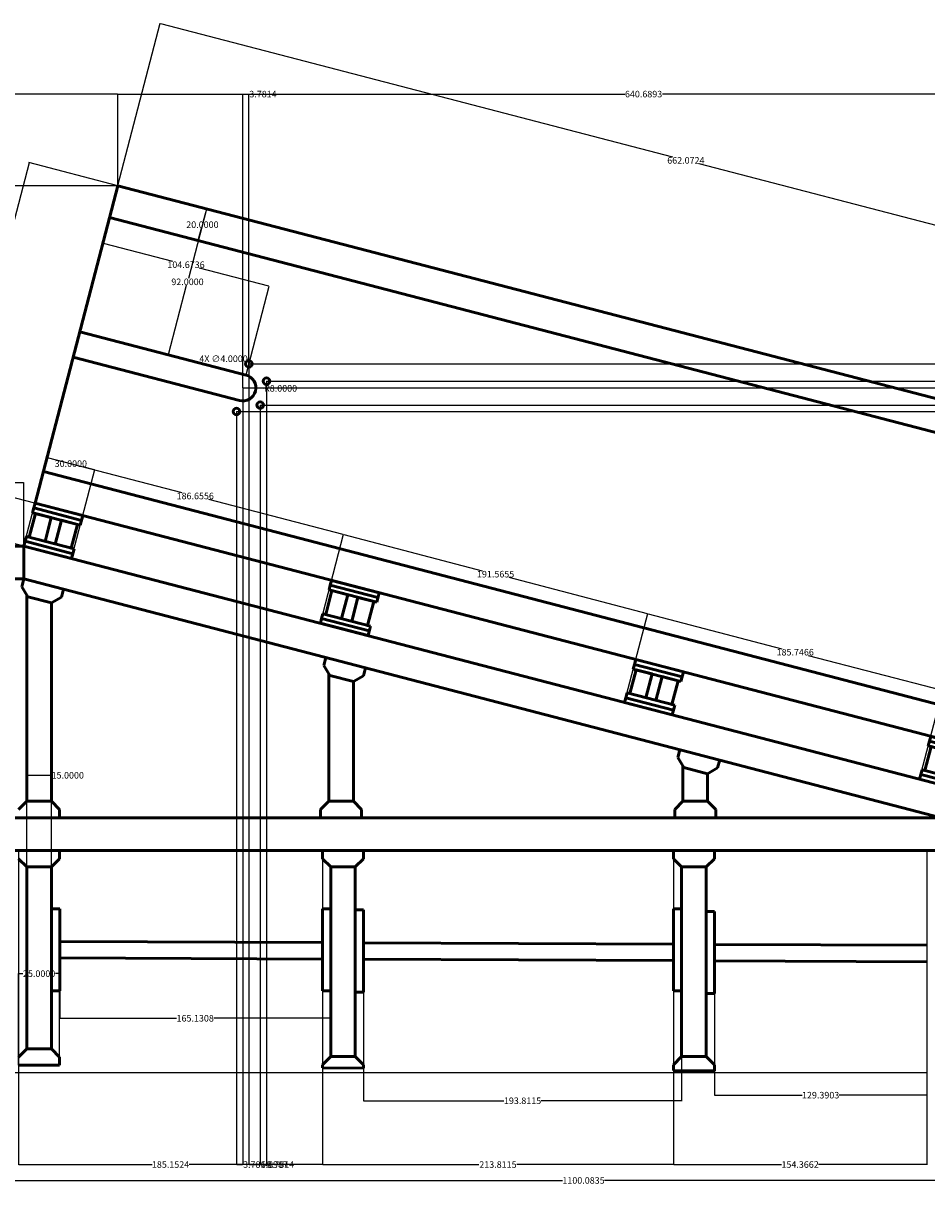
# Model space of a CAD drawing. Units: millimetres. Extents: x -54 to 1187, y -193 to 515.
# Tile 2 of 3: x 222 to 773, y -193 to 515. Entities that reach past the tile are written whole.
import ezdxf

# ---------------------------------------------------------------- set-up
doc = ezdxf.new("R2010")
doc.units = ezdxf.units.MM
doc.header["$MEASUREMENT"] = 0
doc.layers.add('M-DIMS', color=2, linetype='Continuous', lineweight=25)
doc.layers.add('M-OUTL', color=7, linetype='Continuous', lineweight=50)
doc.styles.get("Standard").update_dxf_attribs({"font": 'arial.ttf'})
doc.dimstyles.get("Standard").update_dxf_attribs({"dimtxt": 4, "dimasz": 0.18, "dimexe": 0.18, "dimexo": 0.0625, "dimgap": 0.09, "dimtad": 0, "dimtih": 1, "dimtoh": 1, "dimdec": 4, "dimzin": 0, "dimdsep": 46, "dimtxsty": 'Standard', "dimcen": 0.09, "dimclrd": 3, "dimclre": 3, "dimclrt": 1, "dimadec": 0, "dimazin": 0, "dimtfac": 1, "dimtdec": 4, "dimtofl": 0, "dimtmove": 0, "dimatfit": 3, "dimfxl": 1, "dimtolj": 1, "dimtzin": 0, "dimarcsym": 0})

# ---------------------------------------------------------------- blocks, each defined once
blk = doc.blocks.new('*D1')
at = {"layer": 'Defpoints', "color": 0, "transparency": 16777216}
for p in [(13.68, 20.33), (1113.76, 20.33), (1113.76, -190.81)]:
    blk.add_point(p, dxfattribs=at)
at = {"layer": 'M-DIMS', "color": 0, "lineweight": -2, "transparency": 16777216}
for p, q in [((13.68, 20.27), (13.68, -190.99)), ((1113.76, 20.27), (1113.76, -190.99)), ((13.86, -190.81), (550.84, -190.81)), ((1113.58, -190.81), (576.6, -190.81))]:
    blk.add_line(p, q, dxfattribs=at)
at = {"layer": 'M-DIMS', "color": 0, "transparency": 16777216}
for points in [[(13.86, -190.78), (13.86, -190.84), (13.68, -190.81)], [(1113.58, -190.78), (1113.58, -190.84), (1113.76, -190.81)]]:
    blk.add_solid(points, dxfattribs=at)
at = {"layer": 'M-DIMS', "color": 0, "transparency": 16777216, "insert": (563.72, -190.81), "char_height": 4, "attachment_point": 5}
blk.add_mtext('\\A1;1100.0835', dxfattribs=at)
blk = doc.blocks.new('*D2')
at = {"layer": 'Defpoints', "color": 0, "transparency": 16777216}
for p in [(244.55, -55.15), (409.68, -57.46), (409.68, -91.94)]:
    blk.add_point(p, dxfattribs=at)
at = {"layer": 'M-DIMS', "color": 0, "lineweight": -2, "transparency": 16777216}
for p, q in [((244.55, -55.22), (244.55, -92.12)), ((409.68, -57.52), (409.68, -92.12)), ((244.73, -91.94), (315.8, -91.94)), ((409.5, -91.94), (338.43, -91.94))]:
    blk.add_line(p, q, dxfattribs=at)
at = {"layer": 'M-DIMS', "color": 0, "transparency": 16777216}
for points in [[(244.73, -91.91), (244.73, -91.97), (244.55, -91.94)], [(409.5, -91.91), (409.5, -91.97), (409.68, -91.94)]]:
    blk.add_solid(points, dxfattribs=at)
at = {"layer": 'M-DIMS', "color": 0, "transparency": 16777216, "insert": (327.11, -91.94), "char_height": 4, "attachment_point": 5}
blk.add_mtext('\\A1;165.1308', dxfattribs=at)
blk = doc.blocks.new('*D3')
at = {"layer": 'Defpoints', "color": 0, "transparency": 16777216}
for p in [(429.68, -55.95), (623.49, -55.95), (623.49, -142.23)]:
    blk.add_point(p, dxfattribs=at)
at = {"layer": 'M-DIMS', "color": 0, "lineweight": -2, "transparency": 16777216}
for p, q in [((429.68, -56.02), (429.68, -142.41)), ((623.49, -56.02), (623.49, -142.41)), ((429.86, -142.23), (515.26, -142.23)), ((623.31, -142.23), (537.91, -142.23))]:
    blk.add_line(p, q, dxfattribs=at)
at = {"layer": 'M-DIMS', "color": 0, "transparency": 16777216}
for points in [[(429.86, -142.2), (429.86, -142.26), (429.68, -142.23)], [(623.31, -142.2), (623.31, -142.26), (623.49, -142.23)]]:
    blk.add_solid(points, dxfattribs=at)
at = {"layer": 'M-DIMS', "color": 0, "transparency": 16777216, "insert": (526.58, -142.23), "char_height": 4, "attachment_point": 5}
blk.add_mtext('\\A1;193.8115', dxfattribs=at)
blk = doc.blocks.new('*D4')
at = {"layer": 'Defpoints', "color": 0, "transparency": 16777216}
for p in [(643.49, -51.86), (772.88, -51.86), (772.88, -138.82)]:
    blk.add_point(p, dxfattribs=at)
at = {"layer": 'M-DIMS', "color": 0, "lineweight": -2, "transparency": 16777216}
for p, q in [((643.49, -51.92), (643.49, -139)), ((772.88, -51.92), (772.88, -139)), ((643.67, -138.82), (696.87, -138.82)), ((772.7, -138.82), (719.5, -138.82))]:
    blk.add_line(p, q, dxfattribs=at)
at = {"layer": 'M-DIMS', "color": 0, "transparency": 16777216}
for points in [[(643.67, -138.79), (643.67, -138.85), (643.49, -138.82)], [(772.7, -138.79), (772.7, -138.85), (772.88, -138.82)]]:
    blk.add_solid(points, dxfattribs=at)
at = {"layer": 'M-DIMS', "color": 0, "transparency": 16777216, "insert": (708.19, -138.82), "char_height": 4, "attachment_point": 5}
blk.add_mtext('\\A1;129.3903', dxfattribs=at)
blk = doc.blocks.new('*D5')
at = {"layer": 'Defpoints', "color": 0, "transparency": 16777216}
for p in [(222.75, 234.49), (22.75, 195.91), (222.75, 195.91)]:
    blk.add_point(p, dxfattribs=at)
at = {"layer": 'M-DIMS', "color": 0, "lineweight": -2, "transparency": 16777216}
for p, q in [((22.75, 195.98), (22.75, 234.67)), ((22.93, 234.49), (111.22, 234.49)), ((222.57, 234.49), (134.28, 234.49)), ((222.75, 195.98), (222.75, 234.67))]:
    blk.add_line(p, q, dxfattribs=at)
at = {"layer": 'M-DIMS', "color": 0, "transparency": 16777216}
for points in [[(22.93, 234.52), (22.93, 234.46), (22.75, 234.49)], [(222.57, 234.52), (222.57, 234.46), (222.75, 234.49)]]:
    blk.add_solid(points, dxfattribs=at)
at = {"layer": 'M-DIMS', "color": 0, "transparency": 16777216, "insert": (122.75, 234.49), "char_height": 4, "attachment_point": 5}
blk.add_mtext('\\A1;200.0000', dxfattribs=at)
blk = doc.blocks.new('*D6')
at = {"layer": 'Defpoints', "color": 0, "transparency": 16777216}
for p in [(279.97, 415.58), (946.42, 347.55), (920.66, 248.68)]:
    blk.add_point(p, dxfattribs=at)
at = {"layer": 'M-DIMS', "color": 0, "lineweight": -2, "transparency": 16777216}
for p, q in [((279.99, 415.64), (305.78, 514.63)), ((305.91, 514.41), (617.89, 433.14)), ((946.25, 347.6), (634.26, 428.87)), ((920.68, 248.74), (946.47, 347.73))]:
    blk.add_line(p, q, dxfattribs=at)
at = {"layer": 'M-DIMS', "color": 0, "transparency": 16777216}
for points in [[(305.91, 514.44), (305.9, 514.38), (305.73, 514.46)], [(946.26, 347.63), (946.24, 347.57), (946.42, 347.55)]]:
    blk.add_solid(points, dxfattribs=at)
at = {"layer": 'M-DIMS', "color": 0, "transparency": 16777216, "insert": (626.08, 431.01), "char_height": 4, "attachment_point": 5}
blk.add_mtext('\\A1;662.0724', dxfattribs=at)
blk = doc.blocks.new('ROLLER-BEARING-UNIT')
for p, q in [((5.29, 27.88), (6.05, 30.79)), ((6.81, 33.69), (6.05, 30.79)), ((6.05, 30.79), (35.08, 23.23)), ((35.84, 26.13), (6.81, 33.69)), ((3.24, 12.92), (7.02, 27.44)), ((5.29, 27.88), (34.33, 20.32)), ((7.02, 27.44), (16.7, 24.91)), ((16.7, 24.91), (12.91, 10.4)), ((22.91, 23.3), (19.12, 8.78)), ((32.58, 20.78), (22.91, 23.3)), ((34.33, 20.32), (35.84, 26.13)), ((28.8, 6.26), (32.58, 20.78)), ((0, 7.56), (0.76, 10.47)), ((0, 7.56), (29.03, 0)), ((1.51, 13.37), (0.76, 10.47)), ((0.76, 10.47), (29.79, 2.9)), ((30.54, 5.81), (1.51, 13.37)), ((30.54, 5.81), (28.8, 6.26)), ((29.03, 0), (30.54, 5.81)), ((29.79, 2.9), (29.03, 0))]:
    blk.add_line(p, q)
blk = doc.blocks.new('FLANGE-PLATE')
for p, q in [((0, 50), (0, 0)), ((5, 50), (0, 50)), ((5, 0), (5, 50)), ((0, 0), (5, 0))]:
    blk.add_line(p, q)
blk = doc.blocks.new('*D13')
at = {"layer": 'Defpoints', "color": 0, "transparency": 16777216}
for p in [(-42.17, 415.58), (279.97, 415.58), (772.86, -125.25)]:
    blk.add_point(p, dxfattribs=at)
at = {"layer": 'M-DIMS', "color": 3, "lineweight": -2, "transparency": 16777216}
for p, q in [((279.91, 415.58), (-42.35, 415.58)), ((-42.17, 415.4), (-42.17, 147.3)), ((-42.17, -125.07), (-42.17, 143.03)), ((772.79, -125.25), (-42.35, -125.25))]:
    blk.add_line(p, q, dxfattribs=at)
at = {"layer": 'M-DIMS', "color": 3, "transparency": 16777216}
for points in [[(-42.2, 415.4), (-42.14, 415.4), (-42.17, 415.58)], [(-42.2, -125.07), (-42.14, -125.07), (-42.17, -125.25)]]:
    blk.add_solid(points, dxfattribs=at)
at = {"layer": 'M-DIMS', "color": 1, "transparency": 16777216, "insert": (-42.17, 145.16), "char_height": 4, "attachment_point": 5}
blk.add_mtext('\\A1;540.8329', dxfattribs=at)
blk = doc.blocks.new('*D16')
at = {"layer": 'Defpoints', "color": 0, "transparency": 16777216}
for p in [(219.53, 10.33), (404.68, 10.33), (404.68, -181.1)]:
    blk.add_point(p, dxfattribs=at)
at = {"layer": 'M-DIMS', "color": 3, "lineweight": -2, "transparency": 16777216}
for p, q in [((219.53, 10.27), (219.53, -181.28)), ((404.68, 10.27), (404.68, -181.28)), ((219.71, -181.1), (300.8, -181.1)), ((404.5, -181.1), (323.41, -181.1))]:
    blk.add_line(p, q, dxfattribs=at)
at = {"layer": 'M-DIMS', "color": 3, "transparency": 16777216}
for points in [[(219.71, -181.07), (219.71, -181.13), (219.53, -181.1)], [(404.5, -181.07), (404.5, -181.13), (404.68, -181.1)]]:
    blk.add_solid(points, dxfattribs=at)
at = {"layer": 'M-DIMS', "color": 1, "transparency": 16777216, "insert": (312.1, -181.1), "char_height": 4, "attachment_point": 5}
blk.add_mtext('\\A1;185.1524', dxfattribs=at)
blk = doc.blocks.new('*D17')
at = {"layer": 'Defpoints', "color": 0, "transparency": 16777216}
for p in [(404.68, 10.33), (618.49, 10.33), (618.49, -181.1)]:
    blk.add_point(p, dxfattribs=at)
at = {"layer": 'M-DIMS', "color": 3, "lineweight": -2, "transparency": 16777216}
for p, q in [((404.68, 10.27), (404.68, -181.28)), ((618.49, 10.27), (618.49, -181.28)), ((404.86, -181.1), (500.03, -181.1)), ((618.31, -181.1), (523.13, -181.1))]:
    blk.add_line(p, q, dxfattribs=at)
at = {"layer": 'M-DIMS', "color": 3, "transparency": 16777216}
for points in [[(404.86, -181.07), (404.86, -181.13), (404.68, -181.1)], [(618.31, -181.07), (618.31, -181.13), (618.49, -181.1)]]:
    blk.add_solid(points, dxfattribs=at)
at = {"layer": 'M-DIMS', "color": 1, "transparency": 16777216, "insert": (511.58, -181.1), "char_height": 4, "attachment_point": 5}
blk.add_mtext('\\A1;213.8115', dxfattribs=at)
blk = doc.blocks.new('*D18')
at = {"layer": 'Defpoints', "color": 0, "transparency": 16777216}
for p in [(618.49, 10.33), (772.86, 10.33), (772.86, -181.1)]:
    blk.add_point(p, dxfattribs=at)
at = {"layer": 'M-DIMS', "color": 3, "lineweight": -2, "transparency": 16777216}
for p, q in [((618.49, 10.27), (618.49, -181.28)), ((772.86, 10.27), (772.86, -181.28)), ((618.67, -181.1), (684.38, -181.1)), ((772.68, -181.1), (706.97, -181.1))]:
    blk.add_line(p, q, dxfattribs=at)
at = {"layer": 'M-DIMS', "color": 3, "transparency": 16777216}
for points in [[(618.67, -181.07), (618.67, -181.13), (618.49, -181.1)], [(772.68, -181.07), (772.68, -181.13), (772.86, -181.1)]]:
    blk.add_solid(points, dxfattribs=at)
at = {"layer": 'M-DIMS', "color": 1, "transparency": 16777216, "insert": (695.67, -181.1), "char_height": 4, "attachment_point": 5}
blk.add_mtext('\\A1;154.3662', dxfattribs=at)
blk = doc.blocks.new('*D26')
at = {"layer": 'Defpoints', "color": 0, "transparency": 16777216}
for p in [(244.53, -64.74), (219.53, -120.59), (244.53, -120.59)]:
    blk.add_point(p, dxfattribs=at)
at = {"layer": 'M-DIMS', "color": 3, "lineweight": -2, "transparency": 16777216}
for p, q in [((219.53, -120.53), (219.53, -64.56)), ((219.71, -64.74), (222.05, -64.74)), ((244.35, -64.74), (242, -64.74)), ((244.53, -120.53), (244.53, -64.56))]:
    blk.add_line(p, q, dxfattribs=at)
at = {"layer": 'M-DIMS', "color": 3, "transparency": 16777216}
for points in [[(219.71, -64.71), (219.71, -64.77), (219.53, -64.74)], [(244.35, -64.71), (244.35, -64.77), (244.53, -64.74)]]:
    blk.add_solid(points, dxfattribs=at)
at = {"layer": 'M-DIMS', "color": 1, "transparency": 16777216, "insert": (232.03, -64.74), "char_height": 4, "attachment_point": 5}
blk.add_mtext('\\A1;25.0000', dxfattribs=at)
blk = doc.blocks.new('*D27')
at = {"layer": 'Defpoints', "color": 0, "transparency": 16777216}
for p in [(239.53, 56.18), (224.53, 0.33), (239.53, 0.33)]:
    blk.add_point(p, dxfattribs=at)
at = {"layer": 'M-DIMS', "color": 3, "lineweight": -2, "transparency": 16777216}
for p, q in [((224.53, 0.39), (224.53, 56.36)), ((224.71, 56.18), (239.35, 56.18)), ((239.53, 0.39), (239.53, 56.36)), ((239.53, 56.18), (239.71, 56.18))]:
    blk.add_line(p, q, dxfattribs=at)
at = {"layer": 'M-DIMS', "color": 3, "transparency": 16777216}
for points in [[(224.71, 56.21), (224.71, 56.15), (224.53, 56.18)], [(239.35, 56.21), (239.35, 56.15), (239.53, 56.18)]]:
    blk.add_solid(points, dxfattribs=at)
at = {"layer": 'M-DIMS', "color": 1, "transparency": 16777216, "insert": (249.46, 56.18), "char_height": 4, "attachment_point": 5}
blk.add_mtext('\\A1;15.0000', dxfattribs=at)
blk = doc.blocks.new('*D28')
at = {"layer": 'Defpoints', "color": 0, "transparency": 16777216}
for p in [(279.97, 471.43), (279.97, 415.58), (22.75, 195.91)]:
    blk.add_point(p, dxfattribs=at)
at = {"layer": 'M-DIMS', "color": 3, "lineweight": -2, "transparency": 16777216}
for p, q in [((22.75, 195.98), (22.75, 471.61)), ((22.93, 471.43), (139.83, 471.43)), ((279.79, 471.43), (162.9, 471.43)), ((279.97, 415.64), (279.97, 471.61))]:
    blk.add_line(p, q, dxfattribs=at)
at = {"layer": 'M-DIMS', "color": 3, "transparency": 16777216}
for points in [[(22.93, 471.46), (22.93, 471.4), (22.75, 471.43)], [(279.79, 471.46), (279.79, 471.4), (279.97, 471.43)]]:
    blk.add_solid(points, dxfattribs=at)
at = {"layer": 'M-DIMS', "color": 1, "transparency": 16777216, "insert": (151.36, 471.43), "char_height": 4, "attachment_point": 5}
blk.add_mtext('\\A1;257.2253', dxfattribs=at)
blk = doc.blocks.new('*D29')
at = {"layer": 'Defpoints', "color": 0, "transparency": 16777216}
for p in [(920.66, 471.43), (279.97, 415.58), (920.66, 248.68)]:
    blk.add_point(p, dxfattribs=at)
at = {"layer": 'M-DIMS', "color": 3, "lineweight": -2, "transparency": 16777216}
for p, q in [((279.97, 415.64), (279.97, 471.61)), ((280.15, 471.43), (588.81, 471.43)), ((920.48, 471.43), (611.83, 471.43)), ((920.66, 248.74), (920.66, 471.61))]:
    blk.add_line(p, q, dxfattribs=at)
at = {"layer": 'M-DIMS', "color": 3, "transparency": 16777216}
for points in [[(280.15, 471.46), (280.15, 471.4), (279.97, 471.43)], [(920.48, 471.46), (920.48, 471.4), (920.66, 471.43)]]:
    blk.add_solid(points, dxfattribs=at)
at = {"layer": 'M-DIMS', "color": 1, "transparency": 16777216, "insert": (600.32, 471.43), "char_height": 4, "attachment_point": 5}
blk.add_mtext('\\A1;640.6893', dxfattribs=at)
blk = doc.blocks.new('*D30')
at = {"layer": 'Defpoints', "color": 0, "transparency": 16777216}
for p in [(225.93, 429.66), (279.97, 415.58), (229.56, 222.04)]:
    blk.add_point(p, dxfattribs=at)
at = {"layer": 'M-DIMS', "color": 3, "lineweight": -2, "transparency": 16777216}
for p, q in [((225.88, 429.49), (201.27, 335.02)), ((279.91, 415.6), (225.75, 429.71)), ((175.56, 236.29), (200.16, 330.76)), ((229.5, 222.06), (175.34, 236.17))]:
    blk.add_line(p, q, dxfattribs=at)
at = {"layer": 'M-DIMS', "color": 3, "transparency": 16777216}
for points in [[(225.85, 429.49), (225.91, 429.48), (225.93, 429.66)], [(175.53, 236.3), (175.58, 236.29), (175.51, 236.12)]]:
    blk.add_solid(points, dxfattribs=at)
at = {"layer": 'M-DIMS', "color": 1, "transparency": 16777216, "insert": (200.72, 332.89), "char_height": 4, "attachment_point": 5}
blk.add_mtext('\\A1;200.0000', dxfattribs=at)
blk = doc.blocks.new('*D31')
at = {"layer": 'Defpoints', "color": 0, "transparency": 16777216}
for p in [(279.97, 415.58), (274.93, 396.23), (328.98, 382.15)]:
    blk.add_point(p, dxfattribs=at)
at = {"layer": 'M-DIMS', "color": 3, "lineweight": -2, "transparency": 16777216}
for p, q in [((280.04, 415.57), (334.2, 401.46)), ((333.98, 401.33), (332.06, 393.96)), ((274.99, 396.21), (329.15, 382.1)), ((329.02, 382.32), (330.94, 389.69))]:
    blk.add_line(p, q, dxfattribs=at)
at = {"layer": 'M-DIMS', "color": 3, "transparency": 16777216}
for points in [[(333.95, 401.34), (334, 401.32), (334.02, 401.5)], [(329, 382.33), (329.05, 382.31), (328.98, 382.15)]]:
    blk.add_solid(points, dxfattribs=at)
at = {"layer": 'M-DIMS', "color": 1, "transparency": 16777216, "insert": (331.5, 391.82), "char_height": 4, "attachment_point": 5}
blk.add_mtext('\\A1;20.0000', dxfattribs=at)
blk = doc.blocks.new('*D33')
at = {"layer": 'Defpoints', "color": 0, "transparency": 16777216}
for p in [(417.46, 202.93), (222.75, 195.91), (403.38, 148.88)]:
    blk.add_point(p, dxfattribs=at)
at = {"layer": 'M-DIMS', "color": 3, "lineweight": -2, "transparency": 16777216}
for p, q in [((222.77, 195.97), (236.87, 250.14)), ((237, 249.92), (318.95, 228.58)), ((417.28, 202.98), (335.33, 224.31)), ((403.4, 148.94), (417.5, 203.1))]:
    blk.add_line(p, q, dxfattribs=at)
at = {"layer": 'M-DIMS', "color": 3, "transparency": 16777216}
for points in [[(237, 249.94), (236.99, 249.89), (236.82, 249.96)], [(417.29, 203), (417.27, 202.95), (417.46, 202.93)]]:
    blk.add_solid(points, dxfattribs=at)
at = {"layer": 'M-DIMS', "color": 1, "transparency": 16777216, "insert": (327.14, 226.45), "char_height": 4, "attachment_point": 5}
blk.add_mtext('\\A1;186.6556', dxfattribs=at)
blk = doc.blocks.new('*D34')
at = {"layer": 'Defpoints', "color": 0, "transparency": 16777216}
for p in [(403.38, 148.88), (602.84, 154.64), (588.76, 100.59)]:
    blk.add_point(p, dxfattribs=at)
at = {"layer": 'M-DIMS', "color": 3, "lineweight": -2, "transparency": 16777216}
for p, q in [((403.4, 148.94), (417.51, 203.1)), ((417.64, 202.88), (501.97, 180.91)), ((602.67, 154.68), (518.34, 176.65)), ((588.78, 100.65), (602.89, 154.81))]:
    blk.add_line(p, q, dxfattribs=at)
at = {"layer": 'M-DIMS', "color": 3, "transparency": 16777216}
for points in [[(417.64, 202.91), (417.63, 202.85), (417.46, 202.93)], [(602.67, 154.71), (602.66, 154.65), (602.84, 154.64)]]:
    blk.add_solid(points, dxfattribs=at)
at = {"layer": 'M-DIMS', "color": 1, "transparency": 16777216, "insert": (510.15, 178.78), "char_height": 4, "attachment_point": 5}
blk.add_mtext('\\A1;191.5655', dxfattribs=at)
blk = doc.blocks.new('*D35')
at = {"layer": 'Defpoints', "color": 0, "transparency": 16777216}
for p in [(782.59, 107.81), (588.76, 100.59), (768.51, 53.76)]:
    blk.add_point(p, dxfattribs=at)
at = {"layer": 'M-DIMS', "color": 3, "lineweight": -2, "transparency": 16777216}
for p, q in [((588.78, 100.65), (602.89, 154.81)), ((603.02, 154.59), (684.53, 133.36)), ((782.41, 107.86), (700.9, 129.09)), ((768.52, 53.82), (782.63, 107.98))]:
    blk.add_line(p, q, dxfattribs=at)
at = {"layer": 'M-DIMS', "color": 3, "transparency": 16777216}
for points in [[(603.02, 154.62), (603.01, 154.56), (602.84, 154.64)], [(782.42, 107.88), (782.41, 107.83), (782.59, 107.81)]]:
    blk.add_solid(points, dxfattribs=at)
at = {"layer": 'M-DIMS', "color": 1, "transparency": 16777216, "insert": (692.71, 131.22), "char_height": 4, "attachment_point": 5}
blk.add_mtext('\\A1;185.7466', dxfattribs=at)
blk = doc.blocks.new('*D36')
at = {"layer": 'Defpoints', "color": 0, "transparency": 16777216}
for p in [(265.86, 242.4), (222.75, 195.91), (251.78, 188.35)]:
    blk.add_point(p, dxfattribs=at)
at = {"layer": 'M-DIMS', "color": 3, "lineweight": -2, "transparency": 16777216}
for p, q in [((222.77, 195.97), (236.87, 250.13)), ((237, 249.91), (243.15, 248.31)), ((251.8, 188.41), (265.91, 242.57)), ((265.69, 242.44), (259.53, 244.04))]:
    blk.add_line(p, q, dxfattribs=at)
at = {"layer": 'M-DIMS', "color": 3, "transparency": 16777216}
for points in [[(237.01, 249.94), (237, 249.88), (236.83, 249.96)], [(265.69, 242.47), (265.68, 242.41), (265.86, 242.4)]]:
    blk.add_solid(points, dxfattribs=at)
at = {"layer": 'M-DIMS', "color": 1, "transparency": 16777216, "insert": (251.34, 246.18), "char_height": 4, "attachment_point": 5}
blk.add_mtext('\\A1;30.0000', dxfattribs=at)
blk = doc.blocks.new('*D37')
at = {"layer": 'Defpoints', "color": 0, "transparency": 16777216}
for p in [(175.51, 236.12), (229.56, 222.04), (222.75, 195.91)]:
    blk.add_point(p, dxfattribs=at)
at = {"layer": 'M-DIMS', "color": 3, "lineweight": -2, "transparency": 16777216}
for p, q in [((175.46, 235.95), (172.66, 225.19)), ((229.5, 222.06), (175.34, 236.17)), ((168.75, 210.17), (171.55, 220.92)), ((222.69, 195.93), (168.53, 210.04))]:
    blk.add_line(p, q, dxfattribs=at)
at = {"layer": 'M-DIMS', "color": 3, "transparency": 16777216}
for points in [[(175.44, 235.95), (175.49, 235.94), (175.51, 236.12)], [(168.72, 210.17), (168.78, 210.16), (168.7, 209.99)]]:
    blk.add_solid(points, dxfattribs=at)
at = {"layer": 'M-DIMS', "color": 1, "transparency": 16777216, "insert": (172.11, 223.06), "char_height": 4, "attachment_point": 5}
blk.add_mtext('\\A1;27.0000', dxfattribs=at)
blk = doc.blocks.new('*D38')
at = {"layer": 'Defpoints', "color": 0, "transparency": 16777216}
for p in [(279.97, 415.58), (256.78, 326.55), (310.83, 312.47)]:
    blk.add_point(p, dxfattribs=at)
at = {"layer": 'M-DIMS', "color": 3, "lineweight": -2, "transparency": 16777216}
for p, q in [((280.04, 415.57), (334.2, 401.46)), ((333.98, 401.33), (322.98, 359.12)), ((310.87, 312.65), (321.87, 354.86)), ((256.84, 326.54), (311, 312.43))]:
    blk.add_line(p, q, dxfattribs=at)
at = {"layer": 'M-DIMS', "color": 3, "transparency": 16777216}
for points in [[(333.95, 401.34), (334, 401.32), (334.02, 401.5)], [(310.84, 312.65), (310.9, 312.64), (310.83, 312.47)]]:
    blk.add_solid(points, dxfattribs=at)
at = {"layer": 'M-DIMS', "color": 1, "transparency": 16777216, "insert": (322.42, 356.99), "char_height": 4, "attachment_point": 5}
blk.add_mtext('\\A1;92.0000', dxfattribs=at)
blk = doc.blocks.new('*D39')
at = {"layer": 'Defpoints', "color": 0, "transparency": 16777216}
for p in [(372.15, 354.21), (256.78, 326.55), (358.08, 300.17)]:
    blk.add_point(p, dxfattribs=at)
at = {"layer": 'M-DIMS', "color": 3, "lineweight": -2, "transparency": 16777216}
for p, q in [((256.8, 326.61), (270.91, 380.77)), ((271.04, 380.55), (313.32, 369.54)), ((371.98, 354.26), (329.7, 365.27)), ((358.09, 300.23), (372.2, 354.39))]:
    blk.add_line(p, q, dxfattribs=at)
at = {"layer": 'M-DIMS', "color": 3, "transparency": 16777216}
for points in [[(271.04, 380.58), (271.03, 380.52), (270.86, 380.6)], [(371.99, 354.29), (371.97, 354.23), (372.15, 354.21)]]:
    blk.add_solid(points, dxfattribs=at)
at = {"layer": 'M-DIMS', "color": 1, "transparency": 16777216, "insert": (321.51, 367.41), "char_height": 4, "attachment_point": 5}
blk.add_mtext('\\A1;104.6736', dxfattribs=at)
blk = doc.blocks.new('*D47')
at = {"layer": 'Defpoints', "color": 0, "transparency": 16777216}
for p in [(356.06, 292.42), (352.28, 277.91), (356.06, -181.1)]:
    blk.add_point(p, dxfattribs=at)
at = {"layer": 'M-DIMS', "color": 3, "lineweight": -2, "transparency": 16777216}
for p, q in [((356.06, 292.36), (356.06, -181.28)), ((352.28, 277.85), (352.28, -181.28)), ((352.46, -181.1), (355.88, -181.1)), ((356.06, -181.1), (356.24, -181.1))]:
    blk.add_line(p, q, dxfattribs=at)
at = {"layer": 'M-DIMS', "color": 3, "transparency": 16777216}
for points in [[(352.46, -181.07), (352.46, -181.13), (352.28, -181.1)], [(355.88, -181.07), (355.88, -181.13), (356.06, -181.1)]]:
    blk.add_solid(points, dxfattribs=at)
at = {"layer": 'M-DIMS', "color": 1, "transparency": 16777216, "insert": (364.62, -181.1), "char_height": 4, "attachment_point": 5}
blk.add_mtext('\\A1;3.7814', dxfattribs=at)
blk = doc.blocks.new('*D48')
at = {"layer": 'Defpoints', "color": 0, "transparency": 16777216}
for p in [(359.84, 471.43), (359.84, 306.94), (356.06, 292.42)]:
    blk.add_point(p, dxfattribs=at)
at = {"layer": 'M-DIMS', "color": 3, "lineweight": -2, "transparency": 16777216}
for p, q in [((356.06, 292.49), (356.06, 471.61)), ((356.24, 471.43), (359.66, 471.43)), ((359.84, 307), (359.84, 471.61)), ((359.84, 471.43), (360.02, 471.43))]:
    blk.add_line(p, q, dxfattribs=at)
at = {"layer": 'M-DIMS', "color": 3, "transparency": 16777216}
for points in [[(356.24, 471.46), (356.24, 471.4), (356.06, 471.43)], [(359.66, 471.46), (359.66, 471.4), (359.84, 471.43)]]:
    blk.add_solid(points, dxfattribs=at)
at = {"layer": 'M-DIMS', "color": 1, "transparency": 16777216, "insert": (368.4, 471.43), "char_height": 4, "attachment_point": 5}
blk.add_mtext('\\A1;3.7814', dxfattribs=at)
blk = doc.blocks.new('*D49')
at = {"layer": 'Defpoints', "color": 0, "transparency": 16777216}
for p in [(359.84, 306.94), (366.74, 281.89), (366.74, -181.1)]:
    blk.add_point(p, dxfattribs=at)
at = {"layer": 'M-DIMS', "color": 3, "lineweight": -2, "transparency": 16777216}
for p, q in [((359.84, 306.88), (359.84, -181.28)), ((366.74, 281.83), (366.74, -181.28)), ((360.02, -181.1), (366.56, -181.1)), ((366.74, -181.1), (366.92, -181.1))]:
    blk.add_line(p, q, dxfattribs=at)
at = {"layer": 'M-DIMS', "color": 3, "transparency": 16777216}
for points in [[(360.02, -181.07), (360.02, -181.13), (359.84, -181.1)], [(366.56, -181.07), (366.56, -181.13), (366.74, -181.1)]]:
    blk.add_solid(points, dxfattribs=at)
at = {"layer": 'M-DIMS', "color": 1, "transparency": 16777216, "insert": (375.32, -181.1), "char_height": 4, "attachment_point": 5}
blk.add_mtext('\\A1;6.8987', dxfattribs=at)
blk = doc.blocks.new('*D50')
at = {"layer": 'Defpoints', "color": 0, "transparency": 16777216}
for p in [(370.52, 296.41), (366.74, 281.89), (370.52, -181.1)]:
    blk.add_point(p, dxfattribs=at)
at = {"layer": 'M-DIMS', "color": 3, "lineweight": -2, "transparency": 16777216}
for p, q in [((370.52, 296.34), (370.52, -181.28)), ((366.74, 281.83), (366.74, -181.28)), ((366.92, -181.1), (370.34, -181.1)), ((370.52, -181.1), (370.7, -181.1))]:
    blk.add_line(p, q, dxfattribs=at)
at = {"layer": 'M-DIMS', "color": 3, "transparency": 16777216}
for points in [[(366.92, -181.07), (366.92, -181.13), (366.74, -181.1)], [(370.34, -181.07), (370.34, -181.13), (370.52, -181.1)]]:
    blk.add_solid(points, dxfattribs=at)
at = {"layer": 'M-DIMS', "color": 1, "transparency": 16777216, "insert": (379.08, -181.1), "char_height": 4, "attachment_point": 5}
blk.add_mtext('\\A1;3.7814', dxfattribs=at)
blk = doc.blocks.new('*D51')
at = {"layer": 'Defpoints', "color": 0, "transparency": 16777216}
for p in [(352.28, 277.91), (366.74, 281.89), (1169.7, 281.89)]:
    blk.add_point(p, dxfattribs=at)
at = {"layer": 'M-DIMS', "color": 3, "lineweight": -2, "transparency": 16777216}
for p, q in [((352.34, 277.91), (1169.88, 277.91)), ((366.8, 281.89), (1169.88, 281.89)), ((1169.7, 281.89), (1169.7, 282.07)), ((1169.7, 282.07), (1169.88, 282.07)), ((1169.7, 278.09), (1169.7, 281.71))]:
    blk.add_line(p, q, dxfattribs=at)
at = {"layer": 'M-DIMS', "color": 3, "transparency": 16777216}
for points in [[(1169.67, 281.71), (1169.73, 281.71), (1169.7, 281.89)], [(1169.67, 278.09), (1169.73, 278.09), (1169.7, 277.91)]]:
    blk.add_solid(points, dxfattribs=at)
at = {"layer": 'M-DIMS', "color": 1, "transparency": 16777216, "insert": (1178.26, 282.07), "char_height": 4, "attachment_point": 5}
blk.add_mtext('\\A1;3.9830', dxfattribs=at)
blk = doc.blocks.new('*D52')
at = {"layer": 'Defpoints', "color": 0, "transparency": 16777216}
for p in [(356.06, 292.42), (1169.7, 292.42), (366.74, 281.89)]:
    blk.add_point(p, dxfattribs=at)
at = {"layer": 'M-DIMS', "color": 3, "lineweight": -2, "transparency": 16777216}
for p, q in [((356.12, 292.42), (1169.88, 292.42)), ((1169.7, 292.24), (1169.7, 289.29)), ((1169.7, 282.07), (1169.7, 285.02)), ((366.8, 281.89), (1169.88, 281.89))]:
    blk.add_line(p, q, dxfattribs=at)
at = {"layer": 'M-DIMS', "color": 3, "transparency": 16777216}
for points in [[(1169.67, 292.24), (1169.73, 292.24), (1169.7, 292.42)], [(1169.67, 282.07), (1169.73, 282.07), (1169.7, 281.89)]]:
    blk.add_solid(points, dxfattribs=at)
at = {"layer": 'M-DIMS', "color": 1, "transparency": 16777216, "insert": (1169.7, 287.16), "char_height": 4, "attachment_point": 5}
blk.add_mtext('\\A1;10.5326', dxfattribs=at)
blk = doc.blocks.new('*D53')
at = {"layer": 'Defpoints', "color": 0, "transparency": 16777216}
for p in [(356.06, 292.42), (370.52, 296.41), (1169.7, 296.41)]:
    blk.add_point(p, dxfattribs=at)
at = {"layer": 'M-DIMS', "color": 3, "lineweight": -2, "transparency": 16777216}
for p, q in [((356.12, 292.42), (1169.88, 292.42)), ((370.58, 296.41), (1169.88, 296.41)), ((1169.7, 296.41), (1169.7, 296.59)), ((1169.7, 296.59), (1169.88, 296.59)), ((1169.7, 292.6), (1169.7, 296.23))]:
    blk.add_line(p, q, dxfattribs=at)
at = {"layer": 'M-DIMS', "color": 3, "transparency": 16777216}
for points in [[(1169.67, 296.23), (1169.73, 296.23), (1169.7, 296.41)], [(1169.67, 292.6), (1169.73, 292.6), (1169.7, 292.42)]]:
    blk.add_solid(points, dxfattribs=at)
at = {"layer": 'M-DIMS', "color": 1, "transparency": 16777216, "insert": (1178.26, 296.59), "char_height": 4, "attachment_point": 5}
blk.add_mtext('\\A1;3.9830', dxfattribs=at)
blk = doc.blocks.new('*D54')
at = {"layer": 'Defpoints', "color": 0, "transparency": 16777216}
for p in [(359.84, 306.94), (1169.7, 306.94), (370.52, 296.41)]:
    blk.add_point(p, dxfattribs=at)
at = {"layer": 'M-DIMS', "color": 3, "lineweight": -2, "transparency": 16777216}
for p, q in [((359.9, 306.94), (1169.88, 306.94)), ((1169.7, 306.76), (1169.7, 303.81)), ((1169.7, 296.59), (1169.7, 299.54)), ((370.58, 296.41), (1169.88, 296.41))]:
    blk.add_line(p, q, dxfattribs=at)
at = {"layer": 'M-DIMS', "color": 3, "transparency": 16777216}
for points in [[(1169.67, 306.76), (1169.73, 306.76), (1169.7, 306.94)], [(1169.67, 296.59), (1169.73, 296.59), (1169.7, 296.41)]]:
    blk.add_solid(points, dxfattribs=at)
at = {"layer": 'M-DIMS', "color": 1, "transparency": 16777216, "insert": (1169.7, 301.67), "char_height": 4, "attachment_point": 5}
blk.add_mtext('\\A1;10.5326', dxfattribs=at)
blk = doc.blocks.new('*D55')
at = {"layer": 'Defpoints', "color": 0, "transparency": 16777216}
for p in [(356.06, 292.42), (364.06, 292.2)]:
    blk.add_point(p, dxfattribs=at)
at = {"layer": 'M-DIMS', "color": 3, "lineweight": -2, "transparency": 16777216}
for p, q in [((355.97, 292.42), (356.15, 292.42)), ((356.06, 292.33), (356.06, 292.51)), ((368.85, 292.06), (364.24, 292.19))]:
    blk.add_line(p, q, dxfattribs=at)
at = {"layer": 'M-DIMS', "color": 3, "transparency": 16777216}
blk.add_solid([(364.24, 292.22), (364.23, 292.16), (364.06, 292.2)], dxfattribs=at)
at = {"layer": 'M-DIMS', "color": 1, "transparency": 16777216, "insert": (379.15, 292.06), "char_height": 4, "attachment_point": 5}
blk.add_mtext('\\A1;R8.0000', dxfattribs=at)
blk = doc.blocks.new('*D56')
at = {"layer": 'Defpoints', "color": 0, "transparency": 16777216}
for p in [(359.57, 308.92), (360.11, 304.96)]:
    blk.add_point(p, dxfattribs=at)
at = {"layer": 'M-DIMS', "color": 3, "lineweight": -2, "transparency": 16777216}
for p, q in [((359.23, 310.11), (359.41, 310.11)), ((359.41, 310.11), (359.55, 309.1)), ((359.75, 306.94), (359.93, 306.94)), ((359.84, 306.85), (359.84, 307.03))]:
    blk.add_line(p, q, dxfattribs=at)
at = {"layer": 'M-DIMS', "color": 3, "transparency": 16777216}
blk.add_solid([(359.58, 309.1), (359.52, 309.1), (359.57, 308.92)], dxfattribs=at)
at = {"layer": 'M-DIMS', "color": 1, "transparency": 16777216, "insert": (344.39, 310.11), "char_height": 4, "attachment_point": 5}
blk.add_mtext('\\A1;4X ∅4.0000', dxfattribs=at)

msp = doc.modelspace()

# ---------------------------------------------------------------- linework, layer by layer
at = {"layer": 'M-OUTL'}
for p, q in [((279.97484, 415.5813), (229.55607, 222.04074)), ((920.66417, 248.67693), (279.97484, 415.5813)), ((915.62229, 229.32287), (274.93296, 396.22724)), ((358.07512, 300.16508), (256.78221, 326.55264)), ((354.04162, 284.68183), (252.74871, 311.0694)), ((234.59795, 241.3948), (875.28728, 74.49042)), ((229.55607, 222.04074), (228.79979, 219.13763)), ((258.58716, 214.47792), (229.55607, 222.04074)), ((229.55607, 222.04074), (870.2454, 55.13637)), ((225.98662, 201.26973), (229.76803, 215.78527)), ((228.04351, 216.23452), (228.79979, 219.13763)), ((228.04351, 216.23452), (257.07459, 208.67171)), ((228.79979, 219.13763), (257.83088, 211.57482)), ((229.76803, 215.78527), (239.44505, 213.26433)), ((239.44505, 213.26433), (235.66365, 198.74879)), ((257.07459, 208.67171), (258.58716, 214.47792)), ((245.6557, 211.64641), (241.87429, 197.13087)), ((255.33273, 209.12548), (245.6557, 211.64641)), ((251.55132, 194.60993), (255.33273, 209.12548)), ((222.74954, 195.91276), (223.50582, 198.81587)), ((224.2621, 201.71898), (223.50582, 198.81587)), ((223.50582, 198.81587), (252.53691, 191.25306)), ((253.29319, 194.15617), (224.2621, 201.71898)), ((22.74954, 195.91276), (222.74954, 195.91276)), ((222.74954, 195.91276), (222.74954, 175.91276)), ((781.59027, 50.33057), (222.74954, 195.91276)), ((222.74954, 195.91276), (251.78062, 188.34995)), ((253.29319, 194.15617), (251.55132, 194.60993)), ((251.78062, 188.34995), (253.29319, 194.15617)), ((252.53691, 191.25306), (251.78062, 188.34995)), ((22.74954, 175.91276), (222.74954, 175.91276)), ((222.74954, 175.91276), (221.48907, 171.07425)), ((221.48907, 171.07425), (225.06992, 164.98609)), ((222.74954, 175.91276), (781.59027, 30.33057)), ((222.74954, 175.91276), (246.95604, 169.66414)), ((224.52653, 40.33057), (224.52653, 165.91276)), ((239.52653, 161.25453), (225.06992, 164.98609)), ((239.52653, 161.25453), (245.66195, 164.83451)), ((246.95604, 169.66414), (245.66195, 164.83451)), ((239.52653, 40.33057), (239.52653, 161.25453)), ((406.72839, 127.9849), (405.46792, 123.14638)), ((405.46792, 123.14638), (409.04877, 117.05822)), ((430.93489, 121.73627), (429.64079, 116.90664)), ((408.50538, 40.33057), (408.50538, 117.98209)), ((423.50538, 113.32666), (409.04877, 117.05822)), ((423.50538, 113.32666), (429.64079, 116.90664)), ((423.50538, 40.33057), (423.50538, 113.32666)), ((622.50168, 71.77433), (621.24122, 66.93582)), ((621.24122, 66.93582), (624.82207, 60.84766)), ((646.70819, 65.52571), (645.41409, 60.69608)), ((624.27868, 40.33057), (624.27868, 61.77153)), ((639.27868, 57.1161), (624.82207, 60.84766)), ((639.27868, 57.1161), (645.41409, 60.69608)), ((639.27868, 40.33057), (639.27868, 57.1161)), ((219.52653, 35.33057), (224.52653, 40.33057)), ((224.52653, 40.33057), (239.52653, 40.33057)), ((244.52653, 35.33057), (239.52653, 40.33057)), ((403.50538, 35.33057), (408.50538, 40.33057)), ((408.50538, 40.33057), (423.50538, 40.33057)), ((428.50538, 35.33057), (423.50538, 40.33057)), ((619.27868, 35.33057), (624.27868, 40.33057)), ((624.27868, 40.33057), (639.27868, 40.33057)), ((644.27868, 35.33057), (639.27868, 40.33057)), ((13.67803, 30.33057), (1013.67803, 30.33057)), ((244.52653, 35.33057), (244.52653, 30.33057)), ((403.50538, 30.33057), (403.50538, 35.33057)), ((428.50538, 35.33057), (428.50538, 30.33057)), ((619.27868, 30.33057), (619.27868, 35.33057)), ((644.27868, 35.33057), (644.27868, 30.33057)), ((1013.67803, 10.33057), (13.67803, 10.33057)), ((224.52653, 10.33057), (239.52653, 10.33057)), ((244.52653, 5.33057), (244.52653, 10.33057)), ((404.67896, 10.33057), (404.67896, 5.33057)), ((429.67896, 5.33057), (429.67896, 10.33057)), ((618.4905, 10.33057), (618.4905, 5.33057)), ((643.4905, 5.33057), (643.4905, 10.33057)), ((219.52653, 5.33057), (224.52653, 0.33057)), ((224.52653, -110.5934), (224.52653, 0.33057)), ((224.52653, 0.33057), (239.52653, 0.33057)), ((244.52653, 5.33057), (239.52653, 0.33057)), ((239.52653, -110.5934), (239.52653, 0.33057)), ((404.67896, 5.33057), (409.67896, 0.33057)), ((409.67896, -115.25163), (409.67896, 0.33057)), ((409.67896, 0.33057), (424.67896, 0.33057)), ((429.67896, 5.33057), (424.67896, 0.33057)), ((424.67896, -115.25163), (424.67896, 0.33057)), ((618.4905, 5.33057), (623.4905, 0.33057)), ((623.4905, -115.25163), (623.4905, 0.33057)), ((623.4905, 0.33057), (638.4905, 0.33057)), ((643.4905, 5.33057), (638.4905, 0.33057)), ((638.4905, -115.25163), (638.4905, 0.33057)), ((239.54816, -45.13146), (239.54816, -55.13142)), ((244.54816, -45.15309), (404.67896, -45.84591)), ((424.67896, -45.93244), (424.67896, -55.93253)), ((429.67896, -45.95407), (618.4905, -46.77098)), ((638.4905, -46.85751), (638.4905, -56.8576)), ((643.4905, -46.87914), (772.85666, -47.43885)), ((239.5049, -55.13137), (239.54816, -55.13156)), ((244.54816, -55.15319), (404.67896, -55.846)), ((429.67896, -55.95417), (618.4905, -56.77107)), ((643.4905, -56.87924), (772.85666, -57.43895)), ((219.52653, -115.5934), (224.52653, -110.5934)), ((224.52653, -110.5934), (239.52653, -110.5934)), ((244.52653, -115.5934), (239.52653, -110.5934)), ((244.52653, -115.5934), (244.52653, -120.5934)), ((404.67896, -120.25163), (409.67896, -115.25163)), ((404.67896, -122.08473), (404.67896, -120.25163)), ((409.67896, -115.25163), (424.67896, -115.25163)), ((429.67896, -120.25163), (424.67896, -115.25163)), ((429.67896, -120.25163), (429.67896, -122.2861)), ((618.4905, -120.25163), (623.4905, -115.25163)), ((618.4905, -123.8069), (618.4905, -120.25163)), ((623.4905, -115.25163), (638.4905, -115.25163)), ((643.4905, -120.25163), (638.4905, -115.25163)), ((643.4905, -120.25163), (643.4905, -124.00827)), ((219.52653, -120.5934), (244.52653, -120.5934)), ((404.67896, -122.08473), (429.67896, -122.2861)), ((618.4905, -123.8069), (643.4905, -124.00827))]:
    msp.add_line(p, q, dxfattribs=at)
for centre in [(359.83977, 306.939), (370.5199, 296.40643), (366.73849, 281.89089), (352.27696, 277.90791)]:
    msp.add_circle(centre, 2, dxfattribs=at)
msp.add_arc((356.05837, 292.42346), 8, 255.39855107, 75.39855107, dxfattribs=at)

# ---------------------------------------------------------------- block references
for name, p in [('ROLLER-BEARING-UNIT', (403.383, 141.319)), ('ROLLER-BEARING-UNIT', (588.76146, 93.02652)), ('ROLLER-BEARING-UNIT', (768.50893, 46.20096)), ('FLANGE-PLATE', (239.548, -75.131))]:
    msp.add_blockref(name, p, dxfattribs=at)
at = {"layer": 'M-OUTL', "rotation": 180}
for p in [(409.67912, -25.13188), (429.67912, -25.93293), (623.49066, -25.13188), (643.49066, -26.85799)]:
    msp.add_blockref('FLANGE-PLATE', p, dxfattribs=at)

# ---------------------------------------------------------------- dimensions: what is measured, and where the dimension line sits
at = {"layer": 'M-DIMS'}
dim = msp.add_aligned_dim(p1=(279.97484, 415.5813), p2=(920.66417, 248.67693), distance=102.17685, dimstyle='Standard', override={"dimclrd": 0, "dimclre": 0, "dimclrt": 0}, dxfattribs=at)
dim.commit()
dim.dimension.update_dxf_attribs({"geometry": '*D6', "text_midpoint": (626.07766, 431.00594)})
for base, p1, p2, override, picture, middle in [((279.97484, 471.4313), (22.74954, 195.91276), (279.97484, 415.5813), {"dimdec": 4, "dimlfac": 1, "dimrnd": 0, "dimzin": 0, "dimdsep": 46, "dimlunit": 2}, '*D28', (151.36219, 471.4313)), ((920.66417, 471.4313), (279.97484, 415.5813), (920.66417, 248.67693), {"dimdec": 4, "dimlfac": 1, "dimrnd": 0, "dimzin": 0, "dimdsep": 46, "dimlunit": 2}, '*D29', (600.3195, 471.4313)), ((359.83977, 471.4313), (356.05837, 292.42346), (359.83977, 306.939), {"dimdec": 4, "dimlfac": 1, "dimrnd": 0, "dimzin": 0, "dimdsep": 46, "dimlunit": 2}, '*D48', (368.40309, 471.4313)), ((366.73849, -181.10163), (359.83977, 306.939), (366.73849, 281.89089), {"dimdec": 4, "dimlfac": 1, "dimrnd": 0, "dimzin": 0, "dimdsep": 46, "dimlunit": 2}, '*D49', (375.32227, -181.10163)), ((356.05837, -181.10163), (352.27696, 277.90792), (356.05837, 292.42346), {"dimdec": 4, "dimlfac": 1, "dimrnd": 0, "dimzin": 0, "dimdsep": 46, "dimlunit": 2}, '*D47', (364.62168, -181.10163)), ((370.5199, -181.10163), (366.73849, 281.89089), (370.5199, 296.40643), {"dimdec": 4, "dimlfac": 1, "dimrnd": 0, "dimzin": 0, "dimdsep": 46, "dimlunit": 2}, '*D50', (379.08321, -181.10163)), ((222.74954, 234.49469), (22.74954, 195.91276), (222.74954, 195.91276), {"dimclrd": 0, "dimclre": 0, "dimclrt": 0}, '*D5', (122.74954, 234.49469)), ((239.52653, 56.18057), (224.52653, 0.33057), (239.52653, 0.33057), {"dimdec": 4, "dimlfac": 1, "dimrnd": 0, "dimzin": 0, "dimdsep": 46, "dimlunit": 2}, '*D27', (249.4582, 56.18057)), ((1113.76153, -190.8134), (13.67803, 20.33057), (1113.76153, 20.33057), {"dimclrd": 0, "dimclre": 0, "dimclrt": 0}, '*D1', (563.71978, -190.8134)), ((404.67896, -181.10163), (219.52653, 10.33057), (404.67896, 10.33057), {"dimdec": 4, "dimlfac": 1, "dimrnd": 0, "dimzin": 0, "dimdsep": 46, "dimlunit": 2}, '*D16', (312.10275, -181.10163)), ((618.4905, -181.10163), (404.67896, 10.33057), (618.4905, 10.33057), {"dimdec": 4, "dimlfac": 1, "dimrnd": 0, "dimzin": 0, "dimdsep": 46, "dimlunit": 2}, '*D17', (511.58473, -181.10163)), ((772.85666, -181.10163), (618.4905, 10.33057), (772.85666, 10.33057), {"dimdec": 4, "dimlfac": 1, "dimrnd": 0, "dimzin": 0, "dimdsep": 46, "dimlunit": 2}, '*D18', (695.67358, -181.10163)), ((409.67896, -91.94418), (244.54816, -55.15319), (409.67896, -57.46053), {"dimclrd": 0, "dimclre": 0, "dimclrt": 0}, '*D2', (327.11356, -91.94418)), ((623.4905, -142.23111), (429.67896, -55.95417), (623.4905, -55.95417), {"dimclrd": 0, "dimclre": 0, "dimclrt": 0}, '*D3', (526.58473, -142.23111)), ((772.88081, -138.82183), (643.4905, -51.85756), (772.88081, -51.85756), {"dimclrd": 0, "dimclre": 0, "dimclrt": 0}, '*D4', (708.18566, -138.82183)), ((244.52653, -64.7434), (219.52653, -120.5934), (244.52653, -120.5934), {"dimdec": 4, "dimlfac": 1, "dimrnd": 0, "dimzin": 0, "dimdsep": 46, "dimlunit": 2}, '*D26', (232.02653, -64.7434))]:
    dim = msp.add_linear_dim(base=base, p1=p1, p2=p2, dimstyle='Standard', override=override, dxfattribs=at)
    dim.commit()
    dim.dimension.update_dxf_attribs({"geometry": picture, "text_midpoint": middle})
for base, p1, p2, angle, picture, middle in [((225.92864, 429.66074), (229.55607, 222.04074), (279.97484, 415.5813), 75.39855107, '*D30', (200.71925, 332.89046)), ((-42.17197, 415.5813), (772.85666, -125.25163), (279.97484, 415.5813), 90, '*D13', (-42.17197, 145.16483)), ((310.82841, 312.4732), (279.97484, 415.5813), (256.78221, 326.55264), 255.39855107, '*D38', (322.42472, 356.98753)), ((328.97916, 382.1478), (279.97484, 415.5813), (274.93296, 396.22724), 255.39855107, '*D31', (331.5001, 391.82483)), ((372.15456, 354.21128), (256.78221, 326.55264), (358.07512, 300.16508), 345.39855107, '*D39', (321.5081, 367.40506)), ((1169.69504, 306.939), (370.5199, 296.40643), (359.83977, 306.939), 90, '*D54', (1169.69504, 301.67272)), ((1169.69504, 296.40643), (356.05837, 292.42346), (370.5199, 296.40643), 90, '*D53', (1178.25972, 296.58643)), ((1169.69504, 292.42346), (366.73849, 281.89089), (356.05837, 292.42346), 90, '*D52', (1169.69504, 287.15717)), ((1169.69504, 281.89089), (352.27696, 277.90792), (366.73849, 281.89089), 90, '*D51', (1178.25972, 282.07089)), ((417.45522, 202.93029), (222.74954, 195.91276), (403.38302, 148.8822), 345.40621912, '*D33', (327.13848, 226.44557)), ((265.86006, 242.39615), (222.74954, 195.91276), (251.78062, 188.34995), 345.39855107, '*D36', (251.34452, 246.17756)), ((175.50987, 236.12018), (222.74954, 195.91276), (229.55607, 222.04074), 75.39855107, '*D37', (172.10661, 223.05619)), ((602.84091, 154.63593), (403.38302, 148.8822), (588.76147, 100.58973), 345.39855107, '*D34', (510.15168, 178.78217)), ((782.58839, 107.81036), (588.76147, 100.58973), (768.50895, 53.76416), 345.39855107, '*D35', (692.71465, 131.22315))]:
    dim = msp.add_linear_dim(base=base, p1=p1, p2=p2, angle=angle, dimstyle='Standard', override={"dimdec": 4, "dimlfac": 1, "dimrnd": 0, "dimzin": 0, "dimdsep": 46, "dimlunit": 2}, dxfattribs=at)
    dim.commit()
    dim.dimension.update_dxf_attribs({"geometry": picture, "text_midpoint": middle})
dim = msp.add_diameter_dim_2p(p1=(360.1096, 304.95728), p2=(359.56995, 308.92071), text='4X <>', dimstyle='Standard', override={"dimdec": 4, "dimlfac": 1, "dimrnd": 0, "dimzin": 0, "dimdsep": 46, "dimlunit": 2}, dxfattribs=at)
dim.commit()
dim.dimension.update_dxf_attribs({"geometry": '*D56', "text_midpoint": (344.39453, 310.10974), "dimtype": 163})
dim = msp.add_radius_dim(center=(356.05837, 292.42346), mpoint=(364.0552, 292.19845), dimstyle='Standard', override={"dimdec": 4, "dimlfac": 1, "dimrnd": 0, "dimzin": 0, "dimdsep": 46, "dimlunit": 2}, dxfattribs=at)
dim.commit()
dim.dimension.update_dxf_attribs({"geometry": '*D55', "text_midpoint": (368.8533, 292.06344), "dimtype": 164})

doc.saveas('drawing.dxf')
